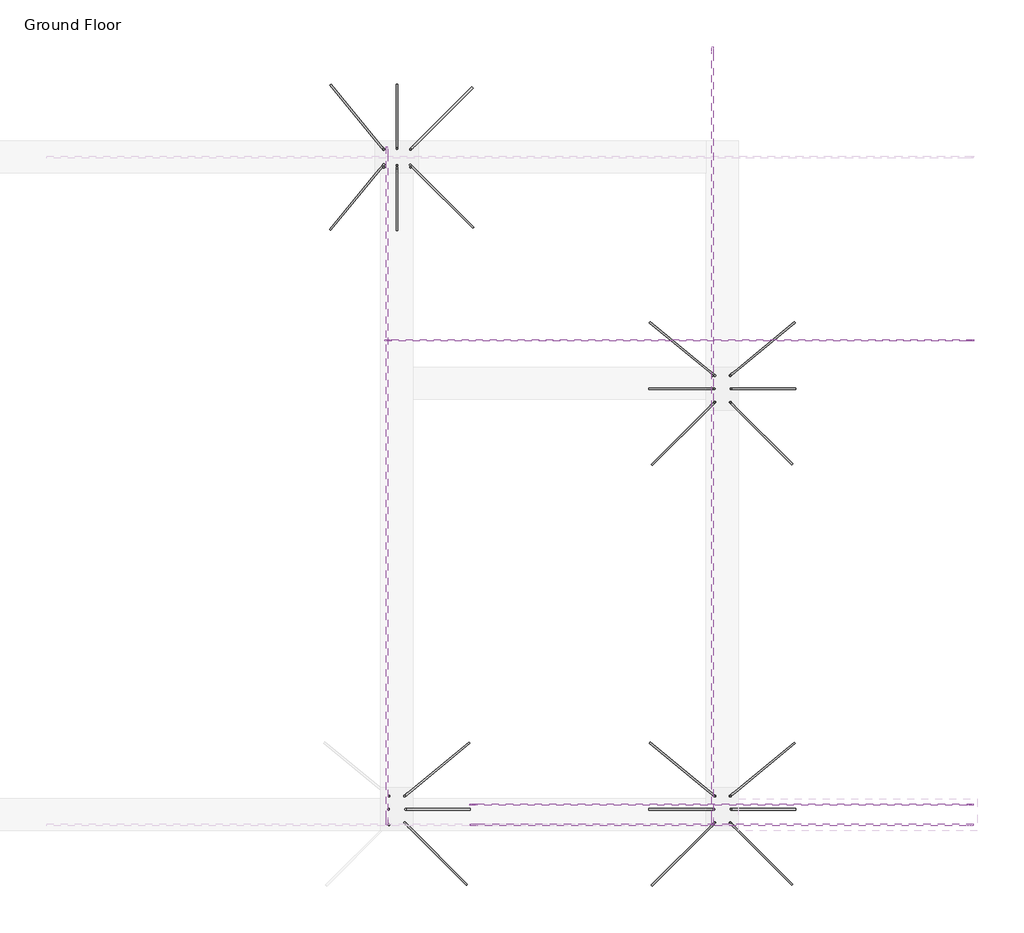
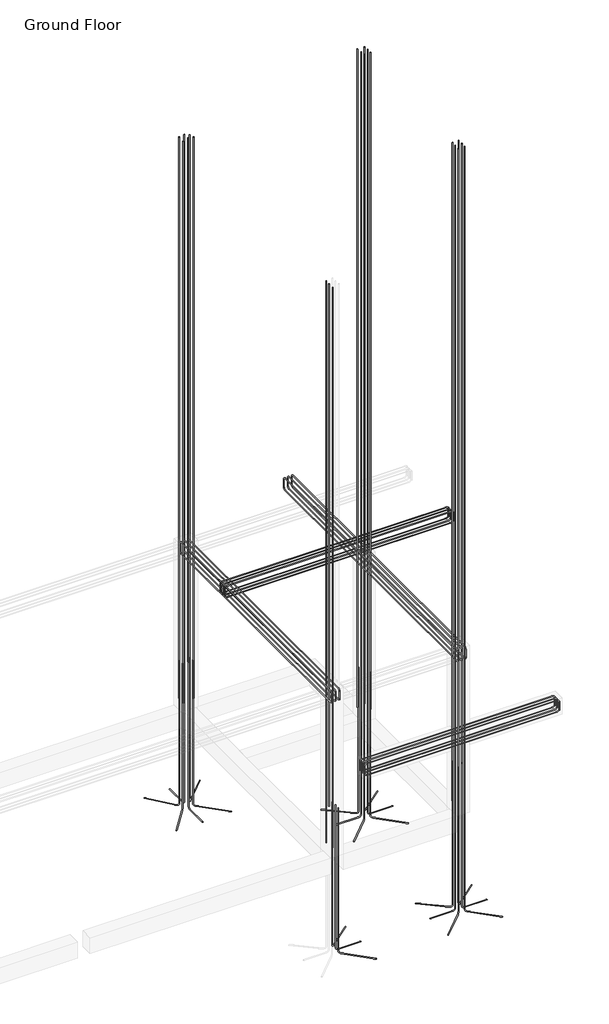
# One storey, part 5 of 5: 50 reinforcing bars.
"""IFC4 building model written with IfcOpenShell, lengths in millimetres."""

from ifc_helpers import new_model, si_unit, point, frame, origin, place, context, project, spatial, polyline, circle_curve, trimmed, segment, composite_curve, source, transform, mapped, element, save
from ifc_brep_helpers import swept_disk

model = new_model("IFC4")

# Units and contexts
model_context = context("Model", 3, world=origin())
ifc_project = project(units=[si_unit("LENGTHUNIT", "METRE", prefix="MILLI")], contexts=[model_context])

# Site, building, storey
site = spatial("IfcSite", under=ifc_project)
building = spatial("IfcBuilding", under=site)
storey = spatial("IfcBuildingStorey", under=building, Name="Ground Floor", Elevation=0.0)

# Reinforcing bars
placement = place(None, origin())
element("IfcReinforcingBar", 1, at=placement, inside=storey, context=model_context, shape_type="SolidModel", body=[
    swept_disk(composite_curve([segment(polyline([(1826.3270087, 244.7072019, 877.2694454), (1826.3270087, 244.7072019, -1868.0)]), True, "CONTINUOUS"), segment(trimmed(circle_curve(frame((1858.8539207, 212.1802899, -1868.0), z_axis=(-0.7071067811865491, -0.707106781186546, 0.0), x_axis=(-32.52691199999981, 32.52691200000001, 0.0)), 46.0), [point((1826.3270087, 244.7072019, -1868.0))], [point((1858.8539207, 212.1802899, -1914.0))], True, "CARTESIAN"), True, "CONTINUOUS"), segment(polyline([(1858.8539207, 212.1802899, -1914.0), (2264.5571801, -193.5229695, -1914.0)]), True, "CONTINUOUS")], self_intersect=False), 6.0),
])
element("IfcReinforcingBar", 2, at=placement, inside=storey, context=model_context, shape_type="SolidModel", body=[
    swept_disk(composite_curve([segment(polyline([(1825.0171723, 432.9867911, 871.8711989), (1825.0171723, 432.9867911, -1868.0)]), True, "CONTINUOUS"), segment(trimmed(circle_curve(frame((1860.5632427, 462.1839978, -1868.0), z_axis=(0.634721884628903, -0.7727406610067401, 0.0), x_axis=(-35.54607039999996, -29.19720669999998, 0.0)), 46.0), [point((1825.0171723, 432.9867911, -1868.0))], [point((1860.5632427, 462.1839978, -1914.0))], True, "CARTESIAN"), True, "CONTINUOUS"), segment(polyline([(1860.5632427, 462.1839978, -1914.0), (2282.8991827, 809.0867522, -1914.0)]), True, "CONTINUOUS")], self_intersect=False), 6.0),
])
element("IfcReinforcingBar", 3, at=placement, inside=storey, context=model_context, shape_type="SolidModel", body=[
    swept_disk(composite_curve([segment(polyline([(1831.9882476, 339.6230123, 875.7528218), (1831.9882476, 339.6230123, -1868.0)]), True, "CONTINUOUS"), segment(trimmed(circle_curve(frame((1877.9882476, 339.6230123, -1868.0), z_axis=(0.0, -1.0, 0.0), x_axis=(-46.0, 0.0, 0.0)), 46.0), [point((1831.9882476, 339.6230123, -1868.0))], [point((1877.9882476, 339.6230123, -1914.0))], True, "CARTESIAN"), True, "CONTINUOUS"), segment(polyline([(1877.9882476, 339.6230123, -1914.0), (2288.9640609, 339.6230123, -1914.0)]), True, "CONTINUOUS")], self_intersect=False), 6.0),
])
element("IfcReinforcingBar", 4, at=placement, inside=storey, context=model_context, shape_type="SolidModel", body=[
    swept_disk(composite_curve([segment(polyline([(1715.4887526, 229.5339681, 10934.0212782), (1715.4887526, 229.5339681, 159.2991411)]), True, "CONTINUOUS")], self_intersect=False), 6.0),
])
element("IfcReinforcingBar", 5, at=placement, inside=storey, context=model_context, shape_type="SolidModel", body=[
    swept_disk(composite_curve([segment(polyline([(1711.3882476, 339.6230123, 892.2840812), (1711.3882476, 339.6230123, 10934.0212782)]), True, "CONTINUOUS")], self_intersect=False), 6.0),
])
element("IfcReinforcingBar", 6, at=placement, inside=storey, context=model_context, shape_type="SolidModel", body=[
    swept_disk(composite_curve([segment(polyline([(1715.4887526, 433.132958, 10938.1538451), (1715.4887526, 433.132958, 134.6074908)]), True, "CONTINUOUS")], self_intersect=False), 6.0),
])
element("IfcReinforcingBar", 7, at=placement, inside=storey, context=model_context, shape_type="SolidModel", body=[
    swept_disk(composite_curve([segment(polyline([(4125.0270087, 244.7072019, 877.2694454), (4125.0270087, 244.7072019, -1868.0)]), True, "CONTINUOUS"), segment(trimmed(circle_curve(frame((4157.5539207, 212.1802899, -1868.0), z_axis=(-0.7071067811865491, -0.707106781186546, 0.0), x_axis=(-32.526912000000266, 32.52691200000001, 0.0)), 46.0), [point((4125.0270087, 244.7072019, -1868.0))], [point((4157.5539207, 212.1802899, -1914.0))], True, "CARTESIAN"), True, "CONTINUOUS"), segment(polyline([(4157.5539207, 212.1802899, -1914.0), (4563.2571801, -193.5229695, -1914.0)]), True, "CONTINUOUS")], self_intersect=False), 6.0),
])
element("IfcReinforcingBar", 8, at=placement, inside=storey, context=model_context, shape_type="SolidModel", body=[
    swept_disk(composite_curve([segment(polyline([(4016.2001029, 245.6611074, 884.8983833), (4016.2001029, 245.6611074, -1868.0)]), True, "CONTINUOUS"), segment(trimmed(circle_curve(frame((3983.673191, 213.1341954, -1868.0), z_axis=(-0.7071067811865491, 0.707106781186546, 0.0), x_axis=(32.52691189999996, 32.52691199999998, 0.0)), 46.0), [point((4016.2001029, 245.6611074, -1868.0))], [point((3983.673191, 213.1341954, -1914.0))], True, "CARTESIAN"), True, "CONTINUOUS"), segment(polyline([(3983.673191, 213.1341954, -1914.0), (3571.5436572, -198.9953384, -1914.0)]), True, "CONTINUOUS")], self_intersect=False), 6.0),
])
element("IfcReinforcingBar", 9, at=placement, inside=storey, context=model_context, shape_type="SolidModel", body=[
    swept_disk(composite_curve([segment(polyline([(4123.7171723, 432.9867911, 871.8711989), (4123.7171723, 432.9867911, -1868.0)]), True, "CONTINUOUS"), segment(trimmed(circle_curve(frame((4159.2632427, 462.1839978, -1868.0), z_axis=(0.634721884628903, -0.7727406610067401, 0.0), x_axis=(-35.546070399999735, -29.19720669999998, 0.0)), 46.0), [point((4123.7171723, 432.9867911, -1868.0))], [point((4159.2632427, 462.1839978, -1914.0))], True, "CARTESIAN"), True, "CONTINUOUS"), segment(polyline([(4159.2632427, 462.1839978, -1914.0), (4581.5991827, 809.0867522, -1914.0)]), True, "CONTINUOUS")], self_intersect=False), 6.0),
])
element("IfcReinforcingBar", 10, at=placement, inside=storey, context=model_context, shape_type="SolidModel", body=[
    swept_disk(composite_curve([segment(polyline([(4017.0160253, 432.7322479, 890.3940928), (4017.0160253, 432.7322479, -1868.0)]), True, "CONTINUOUS"), segment(trimmed(circle_curve(frame((3981.4699549, 461.9294546, -1868.0), z_axis=(0.634721884628903, 0.7727406610067401, 0.0), x_axis=(35.546070399999735, -29.19720669999998, 0.0)), 46.0), [point((4017.0160253, 432.7322479, -1868.0))], [point((3981.4699549, 461.9294546, -1914.0))], True, "CARTESIAN"), True, "CONTINUOUS"), segment(polyline([(3981.4699549, 461.9294546, -1914.0), (3557.3023125, 810.3367522, -1914.0)]), True, "CONTINUOUS")], self_intersect=False), 6.0),
])
element("IfcReinforcingBar", 11, at=placement, inside=storey, context=model_context, shape_type="SolidModel", body=[
    swept_disk(composite_curve([segment(polyline([(4130.6882476, 339.6230123, 875.7528218), (4130.6882476, 339.6230123, -1868.0)]), True, "CONTINUOUS"), segment(trimmed(circle_curve(frame((4176.6882476, 339.6230123, -1868.0), z_axis=(0.0, -1.0, 0.0), x_axis=(-46.0, 0.0, 0.0)), 46.0), [point((4130.6882476, 339.6230123, -1868.0))], [point((4176.6882476, 339.6230123, -1914.0))], True, "CARTESIAN"), True, "CONTINUOUS"), segment(polyline([(4176.6882476, 339.6230123, -1914.0), (4587.6640609, 339.6230123, -1914.0)]), True, "CONTINUOUS")], self_intersect=False), 6.0),
])
element("IfcReinforcingBar", 12, at=placement, inside=storey, context=model_context, shape_type="SolidModel", body=[
    swept_disk(composite_curve([segment(polyline([(4010.0882476, 339.6230123, 879.2840812), (4010.0882476, 339.6230123, -1868.0)]), True, "CONTINUOUS"), segment(trimmed(circle_curve(frame((3964.0882476, 339.6230123, -1868.0), z_axis=(0.0, 1.0, 0.0), x_axis=(46.0, 0.0, 0.0)), 46.0), [point((4010.0882476, 339.6230123, -1868.0))], [point((3964.0882476, 339.6230123, -1914.0))], True, "CARTESIAN"), True, "CONTINUOUS"), segment(polyline([(3964.0882476, 339.6230123, -1914.0), (3550.5777923, 339.6230123, -1914.0)]), True, "CONTINUOUS")], self_intersect=False), 6.0),
])
element("IfcReinforcingBar", 13, at=placement, inside=storey, context=model_context, shape_type="SolidModel", body=[
    swept_disk(composite_curve([segment(polyline([(4126.5877425, 244.5339681, 12794.2305276), (4126.5877425, 244.5339681, 171.0746196)]), True, "CONTINUOUS")], self_intersect=False), 6.0),
])
element("IfcReinforcingBar", 14, at=placement, inside=storey, context=model_context, shape_type="SolidModel", body=[
    swept_disk(composite_curve([segment(polyline([(4130.6882476, 339.6230123, 888.7528218), (4130.6882476, 339.6230123, 12792.7935546)]), True, "CONTINUOUS")], self_intersect=False), 6.0),
])
element("IfcReinforcingBar", 15, at=placement, inside=storey, context=model_context, shape_type="SolidModel", body=[
    swept_disk(composite_curve([segment(polyline([(4126.5877425, 433.132958, 12790.6127039), (4126.5877425, 433.132958, 154.6015232)]), True, "CONTINUOUS")], self_intersect=False), 6.0),
])
element("IfcReinforcingBar", 16, at=placement, inside=storey, context=model_context, shape_type="SolidModel", body=[
    swept_disk(composite_curve([segment(polyline([(4014.1887526, 244.5339681, 12794.2305276), (4014.1887526, 244.5339681, 159.2991411)]), True, "CONTINUOUS")], self_intersect=False), 6.0),
])
element("IfcReinforcingBar", 17, at=placement, inside=storey, context=model_context, shape_type="SolidModel", body=[
    swept_disk(composite_curve([segment(polyline([(4010.0882476, 339.6230123, 892.2840812), (4010.0882476, 339.6230123, 12792.7935546)]), True, "CONTINUOUS")], self_intersect=False), 6.0),
])
element("IfcReinforcingBar", 18, at=placement, inside=storey, context=model_context, shape_type="SolidModel", body=[
    swept_disk(composite_curve([segment(polyline([(4014.1887526, 433.132958, 12790.6127039), (4014.1887526, 433.132958, 134.6074908)]), True, "CONTINUOUS")], self_intersect=False), 6.0),
])
element("IfcReinforcingBar", 19, at=placement, inside=storey, context=model_context, shape_type="SolidModel", body=[
    swept_disk(composite_curve([segment(polyline([(4125.0270087, 3216.5072019, 877.2694454), (4125.0270087, 3216.5072019, -1868.0)]), True, "CONTINUOUS"), segment(trimmed(circle_curve(frame((4157.5539207, 3183.9802899, -1868.0), z_axis=(-0.7071067811865491, -0.7071067811865459, 0.0), x_axis=(-32.526912000000266, 32.52691199999981, 0.0)), 46.0), [point((4125.0270087, 3216.5072019, -1868.0))], [point((4157.5539207, 3183.9802899, -1914.0))], True, "CARTESIAN"), True, "CONTINUOUS"), segment(polyline([(4157.5539207, 3183.9802899, -1914.0), (4563.2571801, 2778.2770305, -1914.0)]), True, "CONTINUOUS")], self_intersect=False), 6.0),
])
element("IfcReinforcingBar", 20, at=placement, inside=storey, context=model_context, shape_type="SolidModel", body=[
    swept_disk(composite_curve([segment(polyline([(4016.2001029, 3217.4611074, 884.8983833), (4016.2001029, 3217.4611074, -1868.0)]), True, "CONTINUOUS"), segment(trimmed(circle_curve(frame((3983.673191, 3184.9341954, -1868.0), z_axis=(-0.7071067811865491, 0.7071067811865459, 0.0), x_axis=(32.52691189999996, 32.52691199999981, 0.0)), 46.0), [point((4016.2001029, 3217.4611074, -1868.0))], [point((3983.673191, 3184.9341954, -1914.0))], True, "CARTESIAN"), True, "CONTINUOUS"), segment(polyline([(3983.673191, 3184.9341954, -1914.0), (3571.5436572, 2772.8046616, -1914.0)]), True, "CONTINUOUS")], self_intersect=False), 6.0),
])
element("IfcReinforcingBar", 21, at=placement, inside=storey, context=model_context, shape_type="SolidModel", body=[
    swept_disk(composite_curve([segment(polyline([(4123.7171723, 3404.7867911, 871.8711989), (4123.7171723, 3404.7867911, -1868.0)]), True, "CONTINUOUS"), segment(trimmed(circle_curve(frame((4159.2632427, 3433.9839978, -1868.0), z_axis=(0.634721884628903, -0.7727406610067401, 0.0), x_axis=(-35.546070399999735, -29.19720670000015, 0.0)), 46.0), [point((4123.7171723, 3404.7867911, -1868.0))], [point((4159.2632427, 3433.9839978, -1914.0))], True, "CARTESIAN"), True, "CONTINUOUS"), segment(polyline([(4159.2632427, 3433.9839978, -1914.0), (4581.5991827, 3780.8867522, -1914.0)]), True, "CONTINUOUS")], self_intersect=False), 6.0),
])
element("IfcReinforcingBar", 22, at=placement, inside=storey, context=model_context, shape_type="SolidModel", body=[
    swept_disk(composite_curve([segment(polyline([(4017.0160253, 3404.5322479, 890.3940928), (4017.0160253, 3404.5322479, -1868.0)]), True, "CONTINUOUS"), segment(trimmed(circle_curve(frame((3981.4699549, 3433.7294546, -1868.0), z_axis=(0.634721884628903, 0.7727406610067401, 0.0), x_axis=(35.546070399999735, -29.197206699999697, 0.0)), 46.0), [point((4017.0160253, 3404.5322479, -1868.0))], [point((3981.4699549, 3433.7294546, -1914.0))], True, "CARTESIAN"), True, "CONTINUOUS"), segment(polyline([(3981.4699549, 3433.7294546, -1914.0), (3557.3023125, 3782.1367522, -1914.0)]), True, "CONTINUOUS")], self_intersect=False), 6.0),
])
element("IfcReinforcingBar", 23, at=placement, inside=storey, context=model_context, shape_type="SolidModel", body=[
    swept_disk(composite_curve([segment(polyline([(4130.6882476, 3311.4230123, 875.7528218), (4130.6882476, 3311.4230123, -1868.0)]), True, "CONTINUOUS"), segment(trimmed(circle_curve(frame((4176.6882476, 3311.4230123, -1868.0), z_axis=(0.0, -1.0, 0.0), x_axis=(-46.0, 0.0, 0.0)), 46.0), [point((4130.6882476, 3311.4230123, -1868.0))], [point((4176.6882476, 3311.4230123, -1914.0))], True, "CARTESIAN"), True, "CONTINUOUS"), segment(polyline([(4176.6882476, 3311.4230123, -1914.0), (4587.6640609, 3311.4230123, -1914.0)]), True, "CONTINUOUS")], self_intersect=False), 6.0),
])
element("IfcReinforcingBar", 24, at=placement, inside=storey, context=model_context, shape_type="SolidModel", body=[
    swept_disk(composite_curve([segment(polyline([(4011.9382476, 3311.4230123, 879.2840812), (4011.9382476, 3311.4230123, -1868.0)]), True, "CONTINUOUS"), segment(trimmed(circle_curve(frame((3965.9382476, 3311.4230123, -1868.0), z_axis=(0.0, 1.0, 0.0), x_axis=(46.0, 0.0, 0.0)), 46.0), [point((4011.9382476, 3311.4230123, -1868.0))], [point((3965.9382476, 3311.4230123, -1914.0))], True, "CARTESIAN"), True, "CONTINUOUS"), segment(polyline([(3965.9382476, 3311.4230123, -1914.0), (3550.5777923, 3311.4230123, -1914.0)]), True, "CONTINUOUS")], self_intersect=False), 6.0),
])
element("IfcReinforcingBar", 25, at=placement, inside=storey, context=model_context, shape_type="SolidModel", body=[
    swept_disk(composite_curve([segment(polyline([(4126.5877425, 3216.3339681, 12794.2305276), (4126.5877425, 3216.3339681, 171.0746196)]), True, "CONTINUOUS")], self_intersect=False), 6.0),
])
element("IfcReinforcingBar", 26, at=placement, inside=storey, context=model_context, shape_type="SolidModel", body=[
    swept_disk(composite_curve([segment(polyline([(4130.6882476, 3311.4230123, 888.7528218), (4130.6882476, 3311.4230123, 12792.7935546)]), True, "CONTINUOUS")], self_intersect=False), 6.0),
])
element("IfcReinforcingBar", 27, at=placement, inside=storey, context=model_context, shape_type="SolidModel", body=[
    swept_disk(composite_curve([segment(polyline([(4126.5877425, 3404.932958, 12790.6127039), (4126.5877425, 3404.932958, 154.6015232)]), True, "CONTINUOUS")], self_intersect=False), 6.0),
])
element("IfcReinforcingBar", 28, at=placement, inside=storey, context=model_context, shape_type="SolidModel", body=[
    swept_disk(composite_curve([segment(polyline([(4014.1887526, 3216.3339681, 12794.2305276), (4014.1887526, 3216.3339681, 159.2991411)]), True, "CONTINUOUS")], self_intersect=False), 6.0),
])
element("IfcReinforcingBar", 29, at=placement, inside=storey, context=model_context, shape_type="SolidModel", body=[
    swept_disk(composite_curve([segment(polyline([(4011.9382476, 3311.4230123, 892.2840812), (4011.9382476, 3311.4230123, 12792.7935546)]), True, "CONTINUOUS")], self_intersect=False), 6.0),
])
element("IfcReinforcingBar", 30, at=placement, inside=storey, context=model_context, shape_type="SolidModel", body=[
    swept_disk(composite_curve([segment(polyline([(3999.1887526, 3404.932958, 12790.6127039), (3999.1887526, 3404.932958, 134.6074908)]), True, "CONTINUOUS")], self_intersect=False), 6.0),
])
element("IfcReinforcingBar", 31, at=placement, inside=storey, context=model_context, shape_type="SolidModel", body=[
    swept_disk(composite_curve([segment(polyline([(1865.8145087, 5003.5722242, 877.2694454), (1865.8145087, 5003.5722242, -1868.0)]), True, "CONTINUOUS"), segment(trimmed(circle_curve(frame((1898.3414207, 5036.0991362, -1868.0), z_axis=(0.7071067811865447, -0.7071067811865503, 0.0), x_axis=(-32.52691200000004, -32.526912000000266, 0.0)), 46.0), [point((1865.8145087, 5003.5722242, -1868.0))], [point((1898.3414207, 5036.0991362, -1914.0))], True, "CARTESIAN"), True, "CONTINUOUS"), segment(polyline([(1898.3414207, 5036.0991362, -1914.0), (2304.0446801, 5441.8023956, -1914.0)]), True, "CONTINUOUS")], self_intersect=False), 6.0),
])
element("IfcReinforcingBar", 32, at=placement, inside=storey, context=model_context, shape_type="SolidModel", body=[
    swept_disk(composite_curve([segment(polyline([(1864.8606033, 4894.7453184, 884.8983833), (1864.8606033, 4894.7453184, -1868.0)]), True, "CONTINUOUS"), segment(trimmed(circle_curve(frame((1897.3875152, 4862.2184065, -1868.0), z_axis=(-0.7071067811865472, -0.7071067811865479, 0.0), x_axis=(-32.52691189999996, 32.526911899999504, 0.0)), 46.0), [point((1864.8606033, 4894.7453184, -1868.0))], [point((1897.3875152, 4862.2184065, -1914.0))], True, "CARTESIAN"), True, "CONTINUOUS"), segment(polyline([(1897.3875152, 4862.2184065, -1914.0), (2309.517049, 4450.0888727, -1914.0)]), True, "CONTINUOUS")], self_intersect=False), 6.0),
])
element("IfcReinforcingBar", 33, at=placement, inside=storey, context=model_context, shape_type="SolidModel", body=[
    swept_disk(composite_curve([segment(polyline([(1677.5349195, 5002.2623878, 871.8711989), (1677.5349195, 5002.2623878, -1868.0)]), True, "CONTINUOUS"), segment(trimmed(circle_curve(frame((1648.3377128, 5037.8084582, -1868.0), z_axis=(0.7727406610067412, 0.6347218846289017, 0.0), x_axis=(29.197206699999924, -35.546070399999735, 0.0)), 46.0), [point((1677.5349195, 5002.2623878, -1868.0))], [point((1648.3377128, 5037.8084582, -1914.0))], True, "CARTESIAN"), True, "CONTINUOUS"), segment(polyline([(1648.3377128, 5037.8084582, -1914.0), (1301.4349584, 5460.1443982, -1914.0)]), True, "CONTINUOUS")], self_intersect=False), 6.0),
])
element("IfcReinforcingBar", 34, at=placement, inside=storey, context=model_context, shape_type="SolidModel", body=[
    swept_disk(composite_curve([segment(polyline([(1677.7894627, 4895.5612408, 890.3940928), (1677.7894627, 4895.5612408, -1868.0)]), True, "CONTINUOUS"), segment(trimmed(circle_curve(frame((1648.592256, 4860.0151704, -1868.0), z_axis=(-0.772740661006739, 0.6347218846289042, 0.0), x_axis=(29.19720670000015, 35.546070399999735, 0.0)), 46.0), [point((1677.7894627, 4895.5612408, -1868.0))], [point((1648.592256, 4860.0151704, -1914.0))], True, "CARTESIAN"), True, "CONTINUOUS"), segment(polyline([(1648.592256, 4860.0151704, -1914.0), (1300.1849584, 4435.8475279, -1914.0)]), True, "CONTINUOUS")], self_intersect=False), 6.0),
])
element("IfcReinforcingBar", 35, at=placement, inside=storey, context=model_context, shape_type="SolidModel", body=[
    swept_disk(composite_curve([segment(polyline([(1770.8986983, 5009.2334631, 875.7528218), (1770.8986983, 5009.2334631, -1868.0)]), True, "CONTINUOUS"), segment(trimmed(circle_curve(frame((1770.8986983, 5055.2334631, -1868.0), z_axis=(1.0, 0.0, 0.0), x_axis=(0.0, -46.0, 0.0)), 46.0), [point((1770.8986983, 5009.2334631, -1868.0))], [point((1770.8986983, 5055.2334631, -1914.0))], True, "CARTESIAN"), True, "CONTINUOUS"), segment(polyline([(1770.8986983, 5055.2334631, -1914.0), (1770.8986983, 5466.2092764, -1914.0)]), True, "CONTINUOUS")], self_intersect=False), 6.0),
])
element("IfcReinforcingBar", 36, at=placement, inside=storey, context=model_context, shape_type="SolidModel", body=[
    swept_disk(composite_curve([segment(polyline([(1770.8986983, 4873.6334631, 879.2840812), (1770.8986983, 4873.6334631, -1868.0)]), True, "CONTINUOUS"), segment(trimmed(circle_curve(frame((1770.8986983, 4827.6334631, -1868.0), z_axis=(-1.0, 0.0, 0.0), x_axis=(0.0, 46.0, 0.0)), 46.0), [point((1770.8986983, 4873.6334631, -1868.0))], [point((1770.8986983, 4827.6334631, -1914.0))], True, "CARTESIAN"), True, "CONTINUOUS"), segment(polyline([(1770.8986983, 4827.6334631, -1914.0), (1770.8986983, 4429.1230078, -1914.0)]), True, "CONTINUOUS")], self_intersect=False), 6.0),
])
element("IfcReinforcingBar", 37, at=placement, inside=storey, context=model_context, shape_type="SolidModel", body=[
    swept_disk(composite_curve([segment(polyline([(1865.9877425, 5005.132958, 10920.626546), (1865.9877425, 5005.132958, 171.0746196)]), True, "CONTINUOUS")], self_intersect=False), 6.0),
])
element("IfcReinforcingBar", 38, at=placement, inside=storey, context=model_context, shape_type="SolidModel", body=[
    swept_disk(composite_curve([segment(polyline([(1770.8986983, 5009.2334631, 888.7528218), (1770.8986983, 5009.2334631, 10954.6841128)]), True, "CONTINUOUS")], self_intersect=False), 6.0),
])
element("IfcReinforcingBar", 39, at=placement, inside=storey, context=model_context, shape_type="SolidModel", body=[
    swept_disk(composite_curve([segment(polyline([(1677.3887526, 5005.132958, 10946.4189789), (1677.3887526, 5005.132958, 154.6015232)]), True, "CONTINUOUS")], self_intersect=False), 6.0),
])
element("IfcReinforcingBar", 40, at=placement, inside=storey, context=model_context, shape_type="SolidModel", body=[
    swept_disk(composite_curve([segment(polyline([(1865.9877425, 4877.7339681, 10957.5617722), (1865.9877425, 4877.7339681, 159.2991411)]), True, "CONTINUOUS")], self_intersect=False), 6.0),
])
element("IfcReinforcingBar", 41, at=placement, inside=storey, context=model_context, shape_type="SolidModel", body=[
    swept_disk(composite_curve([segment(polyline([(1770.8986983, 4890.4834631, 892.2840812), (1770.8986983, 4890.4834631, 10958.8166797)]), True, "CONTINUOUS")], self_intersect=False), 6.0),
])
element("IfcReinforcingBar", 42, at=placement, inside=storey, context=model_context, shape_type="SolidModel", body=[
    swept_disk(composite_curve([segment(polyline([(1677.3887526, 4877.7339681, 10934.0212782), (1677.3887526, 4877.7339681, 134.6074908)]), True, "CONTINUOUS")], self_intersect=False), 6.0),
])
reinforcing_bar_shape = source(origin(), model_context, "Body", "SolidModel", [
    swept_disk(composite_curve([segment(polyline([(1700.4887526, 5017.2334631, 2963.2994949), (1700.4887526, 5017.2334631, 3111.2994949)]), True, "CONTINUOUS"), segment(trimmed(circle_curve(frame((1700.4887526, 4971.2334631, 3111.2994949), z_axis=(1.0, 0.0, 0.0), x_axis=(0.0, 46.0, 0.0)), 46.0), [point((1700.4887526, 5017.2334631, 3111.2994949))], [point((1700.4887526, 4971.2334631, 3157.2994949))], True, "CARTESIAN"), True, "CONTINUOUS"), segment(polyline([(1700.4887526, 4971.2334631, 3157.2994949), (1700.4887526, 278.4334631, 3157.2994949)]), True, "CONTINUOUS"), segment(trimmed(circle_curve(frame((1700.4887526, 278.4334631, 3111.2994949), z_axis=(1.0, 0.0, 0.0), x_axis=(0.0, 0.0, 46.0)), 46.0), [point((1700.4887526, 278.4334631, 3157.2994949))], [point((1700.4887526, 232.4334631, 3111.2994949))], True, "CARTESIAN"), True, "CONTINUOUS"), segment(polyline([(1700.4887526, 232.4334631, 3111.2994949), (1700.4887526, 232.4334631, 2963.2994949)]), True, "CONTINUOUS")], self_intersect=False), 6.0),
])
element("IfcReinforcingBar", 43, at=placement, inside=storey, context=model_context, shape_type="MappedRepresentation", body=[
    mapped(reinforcing_bar_shape, transform((0.0, 0.0, 0.0), x_axis=(1.0, 0.0, 0.0), y_axis=(0.0, 1.0, 0.0), z_axis=(0.0, 0.0, 1.0))),
    mapped(reinforcing_bar_shape, transform((71.1994949, 0.0, 0.0), x_axis=(1.0, 0.0, 0.0), y_axis=(0.0, 1.0, 0.0), z_axis=(0.0, 0.0, 1.0))),
    mapped(reinforcing_bar_shape, transform((142.3989899, 0.0, 0.0), x_axis=(1.0, 0.0, 0.0), y_axis=(0.0, 1.0, 0.0), z_axis=(0.0, 0.0, 1.0))),
])
reinforcing_bar_2_shape = source(origin(), model_context, "Body", "SolidModel", [
    swept_disk(composite_curve([segment(polyline([(1700.4887526, 5017.2334631, 3132.7005051), (1700.4887526, 5017.2334631, 2984.7005051)]), True, "CONTINUOUS"), segment(trimmed(circle_curve(frame((1700.4887526, 4971.2334631, 2984.7005051), z_axis=(-1.0, 0.0, 0.0), x_axis=(0.0, 46.0, 0.0)), 46.0), [point((1700.4887526, 5017.2334631, 2984.7005051))], [point((1700.4887526, 4971.2334631, 2938.7005051))], True, "CARTESIAN"), True, "CONTINUOUS"), segment(polyline([(1700.4887526, 4971.2334631, 2938.7005051), (1700.4887526, 278.4334631, 2938.7005051)]), True, "CONTINUOUS"), segment(trimmed(circle_curve(frame((1700.4887526, 278.4334631, 2984.7005051), z_axis=(-1.0, 0.0, 0.0), x_axis=(0.0, 0.0, -46.0)), 46.0), [point((1700.4887526, 278.4334631, 2938.7005051))], [point((1700.4887526, 232.4334631, 2984.7005051))], True, "CARTESIAN"), True, "CONTINUOUS"), segment(polyline([(1700.4887526, 232.4334631, 2984.7005051), (1700.4887526, 232.4334631, 3132.7005051)]), True, "CONTINUOUS")], self_intersect=False), 6.0),
])
element("IfcReinforcingBar", 44, at=placement, inside=storey, context=model_context, shape_type="MappedRepresentation", body=[
    mapped(reinforcing_bar_2_shape, transform((0.0, 0.0, 0.0), x_axis=(1.0, 0.0, 0.0), y_axis=(0.0, 1.0, 0.0), z_axis=(0.0, 0.0, 1.0))),
    mapped(reinforcing_bar_2_shape, transform((71.1994949, 0.0, 0.0), x_axis=(1.0, 0.0, 0.0), y_axis=(0.0, 1.0, 0.0), z_axis=(0.0, 0.0, 1.0))),
    mapped(reinforcing_bar_2_shape, transform((142.3989899, 0.0, 0.0), x_axis=(1.0, 0.0, 0.0), y_axis=(0.0, 1.0, 0.0), z_axis=(0.0, 0.0, 1.0))),
])
reinforcing_bar_3_shape = source(origin(), model_context, "Body", "SolidModel", [
    swept_disk(composite_curve([segment(polyline([(3999.1887526, 5724.2386934, 2963.2994949), (3999.1887526, 5724.2386934, 3111.2994949)]), True, "CONTINUOUS"), segment(trimmed(circle_curve(frame((3999.1887526, 5678.2386934, 3111.2994949), z_axis=(1.0, 0.0, 0.0), x_axis=(0.0, 46.0, 0.0)), 46.0), [point((3999.1887526, 5724.2386934, 3111.2994949))], [point((3999.1887526, 5678.2386934, 3157.2994949))], True, "CARTESIAN"), True, "CONTINUOUS"), segment(polyline([(3999.1887526, 5678.2386934, 3157.2994949), (3999.1887526, 278.4334631, 3157.2994949)]), True, "CONTINUOUS"), segment(trimmed(circle_curve(frame((3999.1887526, 278.4334631, 3111.2994949), z_axis=(1.0, 0.0, 0.0), x_axis=(0.0, 0.0, 46.0)), 46.0), [point((3999.1887526, 278.4334631, 3157.2994949))], [point((3999.1887526, 232.4334631, 3111.2994949))], True, "CARTESIAN"), True, "CONTINUOUS"), segment(polyline([(3999.1887526, 232.4334631, 3111.2994949), (3999.1887526, 232.4334631, 2963.2994949)]), True, "CONTINUOUS")], self_intersect=False), 6.0),
])
element("IfcReinforcingBar", 45, at=placement, inside=storey, context=model_context, shape_type="MappedRepresentation", body=[
    mapped(reinforcing_bar_3_shape, transform((0.0, 0.0, 0.0), x_axis=(1.0, 0.0, 0.0), y_axis=(0.0, 1.0, 0.0), z_axis=(0.0, 0.0, 1.0))),
    mapped(reinforcing_bar_3_shape, transform((71.1994949, 0.0, 0.0), x_axis=(1.0, 0.0, 0.0), y_axis=(0.0, 1.0, 0.0), z_axis=(0.0, 0.0, 1.0))),
    mapped(reinforcing_bar_3_shape, transform((142.3989899, 0.0, 0.0), x_axis=(1.0, 0.0, 0.0), y_axis=(0.0, 1.0, 0.0), z_axis=(0.0, 0.0, 1.0))),
])
reinforcing_bar_4_shape = source(origin(), model_context, "Body", "SolidModel", [
    swept_disk(composite_curve([segment(polyline([(3999.1887526, 5724.2386934, 3117.7005051), (3999.1887526, 5724.2386934, 2969.7005051)]), True, "CONTINUOUS"), segment(trimmed(circle_curve(frame((3999.1887526, 5678.2386934, 2969.7005051), z_axis=(-1.0, 0.0, 0.0), x_axis=(0.0, 46.0, 0.0)), 46.0), [point((3999.1887526, 5724.2386934, 2969.7005051))], [point((3999.1887526, 5678.2386934, 2923.7005051))], True, "CARTESIAN"), True, "CONTINUOUS"), segment(polyline([(3999.1887526, 5678.2386934, 2923.7005051), (3999.1887526, 278.4334631, 2923.7005051)]), True, "CONTINUOUS"), segment(trimmed(circle_curve(frame((3999.1887526, 278.4334631, 2969.7005051), z_axis=(-1.0, 0.0, 0.0), x_axis=(0.0, 0.0, -46.0)), 46.0), [point((3999.1887526, 278.4334631, 2923.7005051))], [point((3999.1887526, 232.4334631, 2969.7005051))], True, "CARTESIAN"), True, "CONTINUOUS"), segment(polyline([(3999.1887526, 232.4334631, 2969.7005051), (3999.1887526, 232.4334631, 3117.7005051)]), True, "CONTINUOUS")], self_intersect=False), 6.0),
])
element("IfcReinforcingBar", 46, at=placement, inside=storey, context=model_context, shape_type="MappedRepresentation", body=[
    mapped(reinforcing_bar_4_shape, transform((0.0, 0.0, 0.0), x_axis=(1.0, 0.0, 0.0), y_axis=(0.0, 1.0, 0.0), z_axis=(0.0, 0.0, 1.0))),
    mapped(reinforcing_bar_4_shape, transform((71.1994949, 0.0, 0.0), x_axis=(1.0, 0.0, 0.0), y_axis=(0.0, 1.0, 0.0), z_axis=(0.0, 0.0, 1.0))),
    mapped(reinforcing_bar_4_shape, transform((142.3989899, 0.0, 0.0), x_axis=(1.0, 0.0, 0.0), y_axis=(0.0, 1.0, 0.0), z_axis=(0.0, 0.0, 1.0))),
])
reinforcing_bar_5_shape = source(origin(), model_context, "Body", "SolidModel", [
    swept_disk(composite_curve([segment(polyline([(5841.2691711, 3584.0814555, 2961.5520076), (5841.2691711, 3584.0814555, 3109.5520076)]), True, "CONTINUOUS"), segment(trimmed(circle_curve(frame((5795.2691711, 3584.0814555, 3109.5520076), z_axis=(0.0, -1.0, 0.0), x_axis=(46.0, 0.0, 0.0)), 46.0), [point((5841.2691711, 3584.0814555, 3109.5520076))], [point((5795.2691711, 3584.0814555, 3155.5520076))], True, "CARTESIAN"), True, "CONTINUOUS"), segment(polyline([(5795.2691711, 3584.0814555, 3155.5520076), (1734.3882476, 3584.0814555, 3155.5520076)]), True, "CONTINUOUS"), segment(trimmed(circle_curve(frame((1734.3882476, 3584.0814555, 3109.5520076), z_axis=(0.0, -1.0, 0.0), x_axis=(0.0, 0.0, 46.0)), 46.0), [point((1734.3882476, 3584.0814555, 3155.5520076))], [point((1688.3882476, 3584.0814555, 3109.5520076))], True, "CARTESIAN"), True, "CONTINUOUS"), segment(polyline([(1688.3882476, 3584.0814555, 3109.5520076), (1688.3882476, 3584.0814555, 2961.5520076)]), True, "CONTINUOUS")], self_intersect=False), 6.0),
])
element("IfcReinforcingBar", 47, at=placement, inside=storey, context=model_context, shape_type="MappedRepresentation", body=[
    mapped(reinforcing_bar_5_shape, transform((0.0, 0.0, 0.0), x_axis=(1.0, 0.0, 0.0), y_axis=(0.0, 1.0, 0.0), z_axis=(0.0, 0.0, 1.0))),
    mapped(reinforcing_bar_5_shape, transform((0.0, 69.4520076, 0.0), x_axis=(1.0, 0.0, 0.0), y_axis=(0.0, 1.0, 0.0), z_axis=(0.0, 0.0, 1.0))),
    mapped(reinforcing_bar_5_shape, transform((0.0, 138.9040151, 0.0), x_axis=(1.0, 0.0, 0.0), y_axis=(0.0, 1.0, 0.0), z_axis=(0.0, 0.0, 1.0))),
])
reinforcing_bar_6_shape = source(origin(), model_context, "Body", "SolidModel", [
    swept_disk(composite_curve([segment(polyline([(5840.2625116, 3584.0814555, 3134.4479924), (5840.2625116, 3584.0814555, 2986.4479924)]), True, "CONTINUOUS"), segment(trimmed(circle_curve(frame((5794.2625116, 3584.0814555, 2986.4479924), z_axis=(0.0, 1.0, 0.0), x_axis=(46.0, 0.0, 0.0)), 46.0), [point((5840.2625116, 3584.0814555, 2986.4479924))], [point((5794.2625116, 3584.0814555, 2940.4479924))], True, "CARTESIAN"), True, "CONTINUOUS"), segment(polyline([(5794.2625116, 3584.0814555, 2940.4479924), (1734.3882476, 3584.0814555, 2940.4479924)]), True, "CONTINUOUS"), segment(trimmed(circle_curve(frame((1734.3882476, 3584.0814555, 2986.4479924), z_axis=(0.0, 1.0, 0.0), x_axis=(0.0, 0.0, -46.0)), 46.0), [point((1734.3882476, 3584.0814555, 2940.4479924))], [point((1688.3882476, 3584.0814555, 2986.4479924))], True, "CARTESIAN"), True, "CONTINUOUS"), segment(polyline([(1688.3882476, 3584.0814555, 2986.4479924), (1688.3882476, 3584.0814555, 3134.4479924)]), True, "CONTINUOUS")], self_intersect=False), 6.0),
])
element("IfcReinforcingBar", 48, at=placement, inside=storey, context=model_context, shape_type="MappedRepresentation", body=[
    mapped(reinforcing_bar_6_shape, transform((0.0, 0.0, 0.0), x_axis=(1.0, 0.0, 0.0), y_axis=(0.0, 1.0, 0.0), z_axis=(0.0, 0.0, 1.0))),
    mapped(reinforcing_bar_6_shape, transform((0.0, 69.4520076, 0.0), x_axis=(1.0, 0.0, 0.0), y_axis=(0.0, 1.0, 0.0), z_axis=(0.0, 0.0, 1.0))),
    mapped(reinforcing_bar_6_shape, transform((0.0, 138.9040151, 0.0), x_axis=(1.0, 0.0, 0.0), y_axis=(0.0, 1.0, 0.0), z_axis=(0.0, 0.0, 1.0))),
])
reinforcing_bar_7_shape = source(origin(), model_context, "Body", "SolidModel", [
    swept_disk(composite_curve([segment(polyline([(5841.2691711, 229.5339681, 1363.0994949), (5841.2691711, 229.5339681, 1511.0994949)]), True, "CONTINUOUS"), segment(trimmed(circle_curve(frame((5795.2691711, 229.5339681, 1511.0994949), z_axis=(0.0, -1.0, 0.0), x_axis=(46.0, 0.0, 0.0)), 46.0), [point((5841.2691711, 229.5339681, 1511.0994949))], [point((5795.2691711, 229.5339681, 1557.0994949))], True, "CARTESIAN"), True, "CONTINUOUS"), segment(polyline([(5795.2691711, 229.5339681, 1557.0994949), (2337.5636354, 229.5339681, 1557.0994949)]), True, "CONTINUOUS"), segment(trimmed(circle_curve(frame((2337.5636354, 229.5339681, 1511.0994949), z_axis=(0.0, -1.0, 0.0), x_axis=(0.0, 0.0, 46.0)), 46.0), [point((2337.5636354, 229.5339681, 1557.0994949))], [point((2291.5636354, 229.5339681, 1511.0994949))], True, "CARTESIAN"), True, "CONTINUOUS"), segment(polyline([(2291.5636354, 229.5339681, 1511.0994949), (2291.5636354, 229.5339681, 1363.0994949)]), True, "CONTINUOUS")], self_intersect=False), 6.0),
])
element("IfcReinforcingBar", 49, at=placement, inside=storey, context=model_context, shape_type="MappedRepresentation", body=[
    mapped(reinforcing_bar_7_shape, transform((0.0, 0.0, 0.0), x_axis=(1.0, 0.0, 0.0), y_axis=(0.0, 1.0, 0.0), z_axis=(0.0, 0.0, 1.0))),
    mapped(reinforcing_bar_7_shape, transform((0.0, 71.1994949, 0.0), x_axis=(1.0, 0.0, 0.0), y_axis=(0.0, 1.0, 0.0), z_axis=(0.0, 0.0, 1.0))),
    mapped(reinforcing_bar_7_shape, transform((0.0, 142.3989899, 0.0), x_axis=(1.0, 0.0, 0.0), y_axis=(0.0, 1.0, 0.0), z_axis=(0.0, 0.0, 1.0))),
])
reinforcing_bar_8_shape = source(origin(), model_context, "Body", "SolidModel", [
    swept_disk(composite_curve([segment(polyline([(5840.2625116, 229.5339681, 1532.5005051), (5840.2625116, 229.5339681, 1384.5005051)]), True, "CONTINUOUS"), segment(trimmed(circle_curve(frame((5794.2625116, 229.5339681, 1384.5005051), z_axis=(0.0, 1.0, 0.0), x_axis=(46.0, 0.0, 0.0)), 46.0), [point((5840.2625116, 229.5339681, 1384.5005051))], [point((5794.2625116, 229.5339681, 1338.5005051))], True, "CARTESIAN"), True, "CONTINUOUS"), segment(polyline([(5794.2625116, 229.5339681, 1338.5005051), (2341.190873, 229.5339681, 1338.5005051)]), True, "CONTINUOUS"), segment(trimmed(circle_curve(frame((2341.190873, 229.5339681, 1384.5005051), z_axis=(0.0, 1.0, 0.0), x_axis=(0.0, 0.0, -46.0)), 46.0), [point((2341.190873, 229.5339681, 1338.5005051))], [point((2295.190873, 229.5339681, 1384.5005051))], True, "CARTESIAN"), True, "CONTINUOUS"), segment(polyline([(2295.190873, 229.5339681, 1384.5005051), (2295.190873, 229.5339681, 1532.5005051)]), True, "CONTINUOUS")], self_intersect=False), 6.0),
])
element("IfcReinforcingBar", 50, at=placement, inside=storey, context=model_context, shape_type="MappedRepresentation", body=[
    mapped(reinforcing_bar_8_shape, transform((0.0, 0.0, 0.0), x_axis=(1.0, 0.0, 0.0), y_axis=(0.0, 1.0, 0.0), z_axis=(0.0, 0.0, 1.0))),
    mapped(reinforcing_bar_8_shape, transform((0.0, 71.1994949, 0.0), x_axis=(1.0, 0.0, 0.0), y_axis=(0.0, 1.0, 0.0), z_axis=(0.0, 0.0, 1.0))),
    mapped(reinforcing_bar_8_shape, transform((0.0, 142.3989899, 0.0), x_axis=(1.0, 0.0, 0.0), y_axis=(0.0, 1.0, 0.0), z_axis=(0.0, 0.0, 1.0))),
])

save(model, "model.ifc")

# Revit data of these elements
# Elements 1, 2, 3, 4, 5, 6, 7, 8, 9, 10, 11, 12, 13, 14, 15, 16, 17, 18, 19, 20, 21, 22, 23, 24, 25, 26, 27, 28, 29, 30, 31, 32, 33, 34, 35, 36, 37, 38, 39, 40, 41, 42, 43, 44, 45, 46, 47, 48, 49, 50 (IfcReinforcingBar)
#   Phase Created = New Construction
